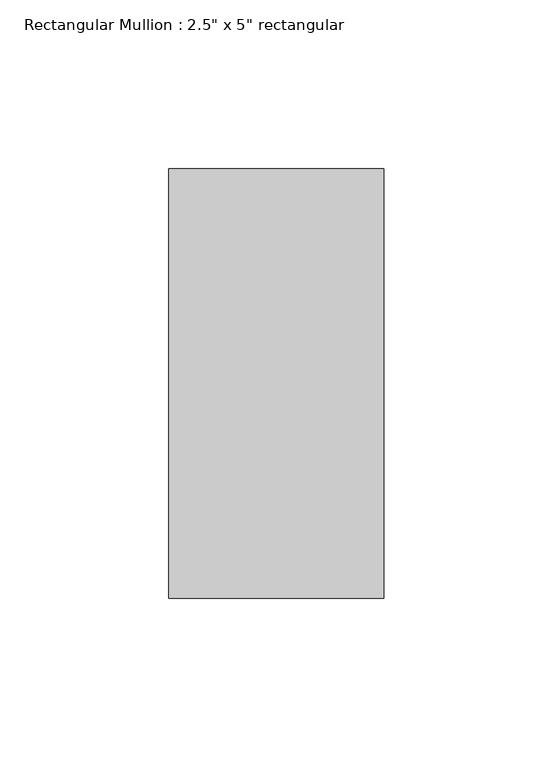
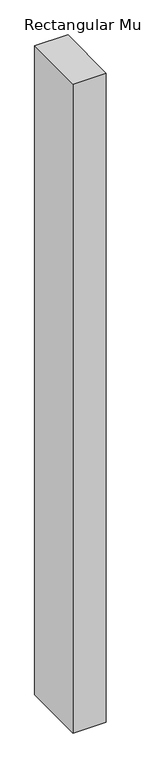
"""IFC4 building model written with IfcOpenShell, lengths in millimetres: member geometry."""

from ifc_helpers import new_model, si_unit, frame, origin, place, context, project, spatial, polyline, outline, extrude, source, transform, mapped, element, save


def member_068505eb(model_context):
    return source(origin(), model_context, "Body", "SweptSolid", [
        extrude(outline(polyline([(0.0, 63.5), (0.0, -63.5), (-63.5, -63.5), (-63.5, 63.5), (0.0, 63.5)])), frame((0.0, 0.0, -1312.0463864), z_axis=(0.0, 0.0, 1.0), x_axis=(1.0, 0.0, 0.0)), (0.0, 0.0, 1.0), 1312.0463864),
    ])


if __name__ == "__main__":
    model = new_model("IFC4")
    model_context = context("Model", 3, world=origin())
    ifc_project = project(units=[si_unit("LENGTHUNIT", "METRE", prefix="MILLI")], contexts=[model_context])
    site = spatial("IfcSite", under=ifc_project)
    building = spatial("IfcBuilding", under=site)
    placement = place(None, origin())
    member_shape = member_068505eb(model_context)
    element("IfcMember", 1, ObjectType="Rectangular Mullion : 2.5\" x 5\" rectangular", at=placement, inside=building, context=model_context, shape_type="MappedRepresentation", body=[
        mapped(member_shape, transform((0.0, 0.0, 0.0), x_axis=(1.0, 0.0, 0.0), y_axis=(0.0, 1.0, 0.0), z_axis=(0.0, 0.0, 1.0))),
    ])
    save(model, "model.ifc")

# Revit data of these elements
# Type "Rectangular Mullion : 2.5\" x 5\" rectangular"
#   built-in parameter 1007304 = 0.416667 (stored number, unit not read)
#   built-in parameter 1007301 = 0.104167 (stored number, unit not read)
#   built-in parameter 1007300 = 0.104167 (stored number, unit not read)
# Element 1 (IfcMember, "Rectangular Mullion : 2.5\" x 5\" rectangular")
#   Materials on its faces: "Aluminum"
# Materials
#   "Aluminum": class "Metal", colour RGB 247 247 247, transparency 0, Description = "Aluminum 6061", Cost = 0
